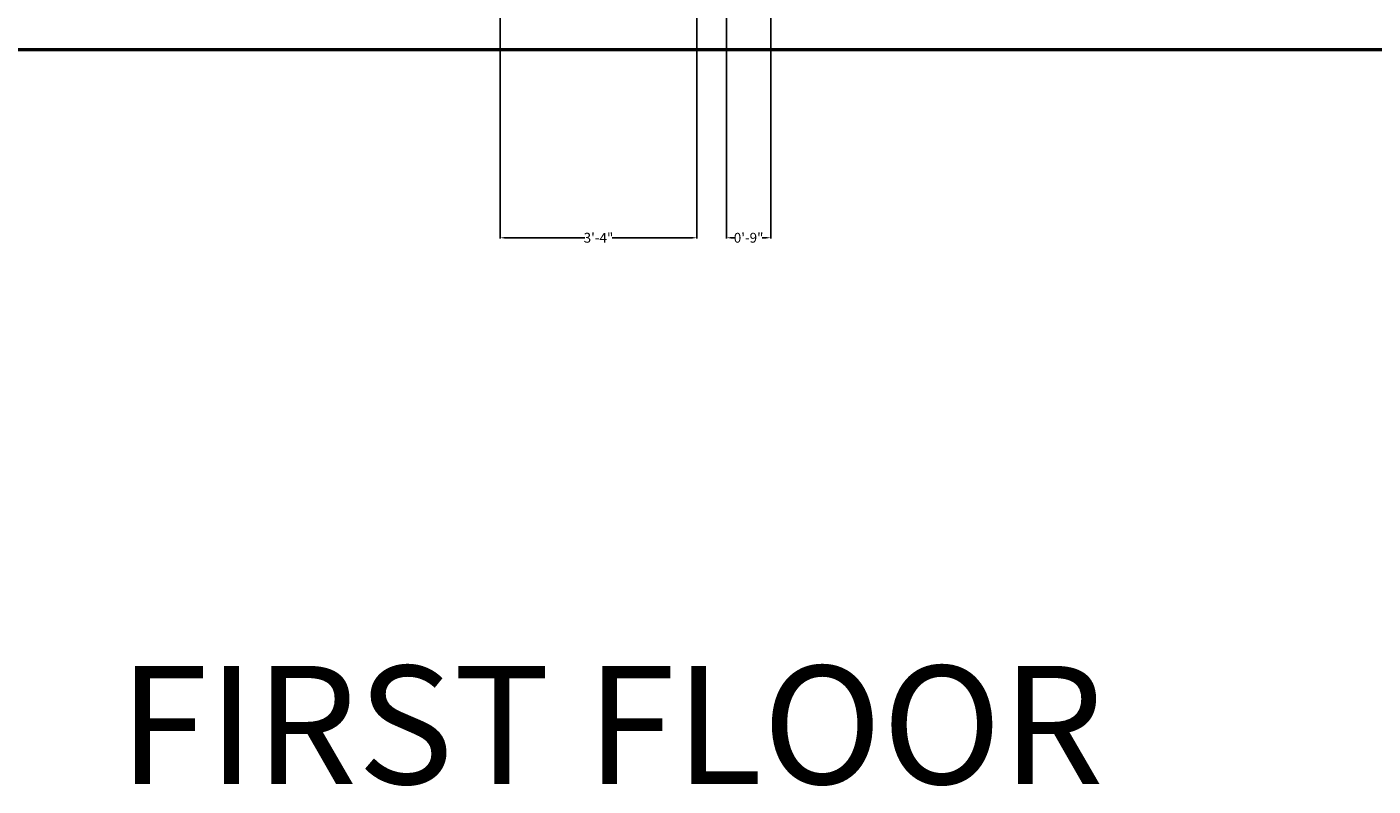
# Model space of a CAD drawing. Units: inches. Extents: x 409 to 7572, y 7 to 725.
# Tile 8 of 38: x 1698 to 1972, y 7 to 161. Entities that reach past the tile are written whole.
import ezdxf

# ---------------------------------------------------------------- set-up
doc = ezdxf.new("R2010")
doc.units = ezdxf.units.IN
doc.header["$MEASUREMENT"] = 0
for name, color, linetype, lineweight in [('A-ANNO-DIMS', 2, 'Continuous', 18), ('A-ANNO-TEXT', 7, 'Continuous', 35), ('A-WALL', 7, 'Continuous', 50)]:
    doc.layers.add(name, color=color, linetype=linetype, lineweight=lineweight)
doc.styles.get("Standard").update_dxf_attribs({"font": 'arial.ttf'})
doc.dimstyles.get("Standard").update_dxf_attribs({"dimtxt": 2, "dimasz": 1, "dimexe": 0.18, "dimexo": 0.0625, "dimgap": 0.09, "dimtad": 0, "dimtih": 1, "dimtoh": 1, "dimdec": 0, "dimzin": 0, "dimdsep": 46, "dimlunit": 3, "dimtxsty": 'Standard', "dimcen": 0.09, "dimadec": 0, "dimazin": 0, "dimtfac": 1, "dimtdec": 0, "dimtofl": 0, "dimtmove": 0, "dimatfit": 3, "dimfxl": 1, "dimtolj": 1, "dimtzin": 0, "dimarcsym": 0})

# ---------------------------------------------------------------- blocks, each defined once
blk = doc.blocks.new('*D179')
at = {"layer": 'A-ANNO-DIMS', "color": 0, "lineweight": -2, "transparency": 16777216}
for p, q in [((1840.32, 165.47), (1840.32, 118.1)), ((1849.32, 165.47), (1849.32, 118.1)), ((1841.32, 118.28), (1842.07, 118.28)), ((1848.32, 118.28), (1847.57, 118.28))]:
    blk.add_line(p, q, dxfattribs=at)
at = {"layer": 'A-ANNO-DIMS', "color": 0, "transparency": 16777216}
for points in [[(1841.32, 118.45), (1841.32, 118.11), (1840.32, 118.28)], [(1848.32, 118.45), (1848.32, 118.11), (1849.32, 118.28)]]:
    blk.add_solid(points, dxfattribs=at)
at = {"layer": 'DEFPOINTS', "color": 0, "transparency": 16777216}
for p in [(1840.32, 165.53), (1849.32, 165.53), (1849.32, 118.28)]:
    blk.add_point(p, dxfattribs=at)
at = {"layer": 'A-ANNO-DIMS', "color": 0, "transparency": 16777216, "insert": (1844.82, 118.28), "char_height": 2, "attachment_point": 5}
blk.add_mtext('\\A1;0\'-9"', dxfattribs=at)
blk = doc.blocks.new('*D182')
at = {"layer": 'A-ANNO-DIMS', "color": 0, "lineweight": -2, "transparency": 16777216}
for p, q in [((1794.32, 170.47), (1794.32, 118.1)), ((1834.32, 170.47), (1834.32, 118.1)), ((1795.32, 118.28), (1811.57, 118.28)), ((1833.32, 118.28), (1817.07, 118.28))]:
    blk.add_line(p, q, dxfattribs=at)
at = {"layer": 'A-ANNO-DIMS', "color": 0, "transparency": 16777216}
for points in [[(1795.32, 118.45), (1795.32, 118.11), (1794.32, 118.28)], [(1833.32, 118.45), (1833.32, 118.11), (1834.32, 118.28)]]:
    blk.add_solid(points, dxfattribs=at)
at = {"layer": 'DEFPOINTS', "color": 0, "transparency": 16777216}
for p in [(1794.32, 170.53), (1834.32, 170.53), (1834.32, 118.28)]:
    blk.add_point(p, dxfattribs=at)
at = {"layer": 'A-ANNO-DIMS', "color": 0, "transparency": 16777216, "insert": (1814.32, 118.28), "char_height": 2, "attachment_point": 5}
blk.add_mtext('\\A1;3\'-4"', dxfattribs=at)

msp = doc.modelspace()

# ---------------------------------------------------------------- linework, layer by layer
at = {"layer": 'A-WALL'}
msp.add_line((1696.32, 156.53), (2070.32, 156.53), dxfattribs=at)

# ---------------------------------------------------------------- texts
at = {"layer": 'A-ANNO-TEXT', "insert": (1716.87, 31.31), "char_height": 24, "attachment_point": 1}
msp.add_mtext_dynamic_manual_height_columns('FIRST FLOOR', width=577.2242, gutter_width=1, heights=[0], dxfattribs=at)

# ---------------------------------------------------------------- dimensions: what is measured, and where the dimension line sits
at = {"layer": 'A-ANNO-DIMS'}
for base, p1, p2, picture, middle in [((1834.32, 118.28), (1794.32, 170.53), (1834.32, 170.53), '*D182', (1814.32, 118.28)), ((1849.32, 118.28), (1840.32, 165.53), (1849.32, 165.53), '*D179', (1844.82, 118.28))]:
    dim = msp.add_linear_dim(base=base, p1=p1, p2=p2, dimstyle='Standard', override={"dimdec": 1, "dimlfac": 1, "dimrnd": 0, "dimzin": 1, "dimdsep": 46, "dimlunit": 4, "dimfrac": 2}, dxfattribs=at)
    dim.commit()
    dim.dimension.update_dxf_attribs({"geometry": picture, "text_midpoint": middle})

doc.saveas('drawing.dxf')
